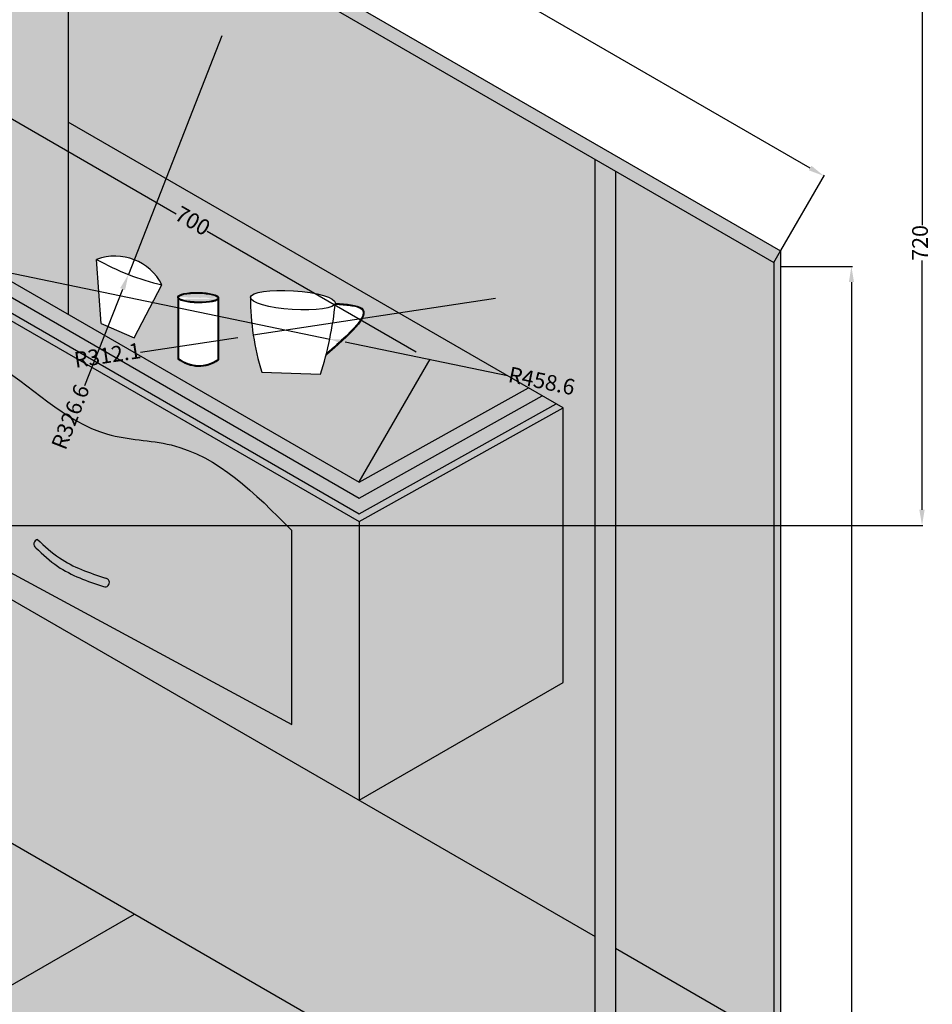
# Model space of a CAD drawing. Units: millimetres. Extents: x 78378 to 86415, y 148682 to 152721.
# Tile 15 of 18: x 80806 to 81968, y 150495 to 151749. Entities that reach past the tile are written whole.
import ezdxf

# ---------------------------------------------------------------- set-up
doc = ezdxf.new("R2010")
doc.units = ezdxf.units.MM
for name, color, linetype, lineweight in [('A-ANNO-DIMS', 2, 'Continuous', 18), ('A-FURN', 4, 'Continuous', 25), ('A-FURN-PATT', 32, 'Continuous', 13)]:
    doc.layers.add(name, color=color, linetype=linetype, lineweight=lineweight)
doc.styles.get("Standard").update_dxf_attribs({"font": 'arial.ttf'})
doc.dimstyles.new('ISO-25', dxfattribs={"dimtxt": 20, "dimasz": 20, "dimexe": 1.25, "dimexo": 0.625, "dimtad": 0, "dimdec": 1, "dimtxsty": 'Standard', "dimcen": 2.5, "dimadec": 0, "dimazin": 0, "dimtfac": 1, "dimtdec": 1, "dimtmove": 0, "dimatfit": 3, "dimfxl": 1, "dimarcsym": 0})

# ---------------------------------------------------------------- blocks, each defined once
blk = doc.blocks.new('*D1')
at = {"layer": 'A-ANNO-DIMS', "color": 0, "lineweight": -2, "transparency": 16777216}
for p, q in [((81775.8, 151435), (81866.6, 151435)), ((81865.3, 151415), (81865.3, 150363.7)), ((81865.3, 149279), (81865.3, 150302.4)), ((81775.8, 149259), (81866.6, 149259))]:
    blk.add_line(p, q, dxfattribs=at)
at = {"layer": 'A-ANNO-DIMS', "color": 0, "transparency": 16777216}
for points in [[(81862, 151415), (81868.6, 151415), (81865.3, 151435)], [(81862, 149279), (81868.6, 149279), (81865.3, 149259)]]:
    blk.add_solid(points, dxfattribs=at)
at = {"layer": 'Defpoints', "color": 0, "transparency": 16777216}
for p in [(81775.2, 151435), (81775.2, 149259), (81865.3, 149259)]:
    blk.add_point(p, dxfattribs=at)
at = {"layer": 'A-ANNO-DIMS', "color": 0, "transparency": 16777216, "insert": (81865.3, 150333), "char_height": 20, "attachment_point": 5, "rotation": 90}
blk.add_mtext('2176', dxfattribs=at)
blk = doc.blocks.new('*D3')
at = {"layer": 'A-ANNO-DIMS', "color": 0, "lineweight": -2, "transparency": 16777216}
for p, q in [((80389.8, 152255.5), (80445.2, 152351.4)), ((80461.9, 152340.3), (81144.7, 151946.1)), ((81812.9, 151560.3), (81195.8, 151916.6)), ((81775.5, 151455.5), (81830.8, 151551.4))]:
    blk.add_line(p, q, dxfattribs=at)
at = {"layer": 'A-ANNO-DIMS', "color": 0, "transparency": 16777216}
for points in [[(80463.5, 152343.2), (80460.2, 152337.4), (80444.5, 152350.3)], [(81814.5, 151563.2), (81811.2, 151557.4), (81830.2, 151550.3)]]:
    blk.add_solid(points, dxfattribs=at)
at = {"layer": 'Defpoints', "color": 0, "transparency": 16777216}
for p in [(80389.5, 152255), (81830.2, 151550.3), (81775.2, 151455)]:
    blk.add_point(p, dxfattribs=at)
at = {"layer": 'A-ANNO-DIMS', "color": 0, "transparency": 16777216, "insert": (81170.2, 151931.4), "char_height": 20, "attachment_point": 5, "rotation": 330}
blk.add_mtext('1600', dxfattribs=at)
blk = doc.blocks.new('*D30')
at = {"layer": 'A-ANNO-DIMS', "color": 0, "lineweight": -2, "transparency": 16777216}
for p, q in [((80615.3, 151825), (81956.4, 151825)), ((81955.2, 151805), (81955.2, 151487.6)), ((81955.2, 151125), (81955.2, 151442.4)), ((80615.3, 151105), (81956.4, 151105))]:
    blk.add_line(p, q, dxfattribs=at)
at = {"layer": 'A-ANNO-DIMS', "color": 0, "transparency": 16777216}
for points in [[(81951.8, 151805), (81958.5, 151805), (81955.2, 151825)], [(81951.8, 151125), (81958.5, 151125), (81955.2, 151105)]]:
    blk.add_solid(points, dxfattribs=at)
at = {"layer": 'Defpoints', "color": 0, "transparency": 16777216}
for p in [(80614.7, 151825), (81955.2, 151825), (80614.7, 151105)]:
    blk.add_point(p, dxfattribs=at)
at = {"layer": 'A-ANNO-DIMS', "color": 0, "transparency": 16777216, "insert": (81955.2, 151465), "char_height": 20, "attachment_point": 5, "rotation": 90}
blk.add_mtext('720', dxfattribs=at)
blk = doc.blocks.new('*D31')
at = {"layer": 'A-ANNO-DIMS', "color": 0, "lineweight": -2, "transparency": 16777216}
for p, q in [((80632.3, 151510.5), (80722.6, 151667)), ((80739.3, 151655.9), (81005.5, 151502.2)), ((81310.9, 151325.9), (81044.7, 151479.6)), ((81238.5, 151160.5), (81328.8, 151317))]:
    blk.add_line(p, q, dxfattribs=at)
at = {"layer": 'A-ANNO-DIMS', "color": 0, "transparency": 16777216}
for points in [[(80741, 151658.8), (80737.7, 151653), (80722, 151665.9)], [(81312.6, 151328.8), (81309.2, 151323), (81328.2, 151315.9)]]:
    blk.add_solid(points, dxfattribs=at)
at = {"layer": 'Defpoints', "color": 0, "transparency": 16777216}
for p in [(80632, 151510), (81328.2, 151315.9), (81238.2, 151160)]:
    blk.add_point(p, dxfattribs=at)
at = {"layer": 'A-ANNO-DIMS', "color": 0, "transparency": 16777216, "insert": (81025.1, 151490.9), "char_height": 20, "attachment_point": 5, "rotation": 330}
blk.add_mtext('700', dxfattribs=at)
blk = doc.blocks.new('*D69')
at = {"layer": 'A-ANNO-DIMS', "color": 0, "lineweight": -2, "transparency": 16777216}
for p, q in [((80751.9, 151435.6), (81200.9, 151342.5)), ((81427.3, 151295.6), (81220.5, 151338.5))]:
    blk.add_line(p, q, dxfattribs=at)
at = {"layer": 'A-ANNO-DIMS', "color": 0, "transparency": 16777216}
blk.add_solid([(81221.2, 151341.8), (81219.8, 151335.2), (81200.9, 151342.5)], dxfattribs=at)
at = {"layer": 'Defpoints', "color": 0, "transparency": 16777216}
for p in [(80751.9, 151435.6), (81200.9, 151342.5)]:
    blk.add_point(p, dxfattribs=at)
at = {"layer": 'A-ANNO-DIMS', "color": 0, "transparency": 16777216, "insert": (81470.4, 151286.7), "char_height": 20, "attachment_point": 5, "rotation": 348.2906}
blk.add_mtext('R458.6', dxfattribs=at)
blk = doc.blocks.new('*D70')
at = {"layer": 'A-ANNO-DIMS', "color": 0, "lineweight": -2, "transparency": 16777216}
for p, q in [((81063.6, 151728.9), (80944.5, 151424.8)), ((80889.1, 151283.3), (80937.2, 151406.2))]:
    blk.add_line(p, q, dxfattribs=at)
at = {"layer": 'A-ANNO-DIMS', "color": 0, "transparency": 16777216}
blk.add_solid([(80934.1, 151407.4), (80940.3, 151405), (80944.5, 151424.8)], dxfattribs=at)
at = {"layer": 'Defpoints', "color": 0, "transparency": 16777216}
for p in [(81063.6, 151728.9), (80944.5, 151424.8)]:
    blk.add_point(p, dxfattribs=at)
at = {"layer": 'A-ANNO-DIMS', "color": 0, "transparency": 16777216, "insert": (80873, 151242.4), "char_height": 20, "attachment_point": 5, "rotation": 68.6084}
blk.add_mtext('R326.6', dxfattribs=at)
blk = doc.blocks.new('*D71')
at = {"layer": 'A-ANNO-DIMS', "color": 0, "lineweight": -2, "transparency": 16777216}
for p, q in [((81412.1, 151394), (81103.5, 151347.4)), ((80959.9, 151325.7), (81083.7, 151344.4))]:
    blk.add_line(p, q, dxfattribs=at)
at = {"layer": 'A-ANNO-DIMS', "color": 0, "transparency": 16777216}
blk.add_solid([(81083.2, 151347.7), (81084.2, 151341.1), (81103.5, 151347.4)], dxfattribs=at)
at = {"layer": 'Defpoints', "color": 0, "transparency": 16777216}
for p in [(81412.1, 151394), (81103.5, 151347.4)]:
    blk.add_point(p, dxfattribs=at)
at = {"layer": 'A-ANNO-DIMS', "color": 0, "transparency": 16777216, "insert": (80918.3, 151319.4), "char_height": 20, "attachment_point": 5, "rotation": 8.593}
blk.add_mtext('R312.1', dxfattribs=at)

msp = doc.modelspace()

# ---------------------------------------------------------------- hatches: boundary and pattern name
at = {"layer": 'A-FURN-PATT'}
h = msp.add_hatch(color=256, dxfattribs=at)
h.dxf.hatch_style = 1
h.paths.add_polyline_path([(78839.3276, 151040.0076), (78579.52, 151190.0076), (78579.52, 150470.0076), (78839.3276, 150320.0076)])
h.paths.add_polyline_path([(79073.1545, 150899.6469, 0.277779695), (79002.2645, 150996.3205, 0.791083931), (78917.9567, 150978.8719, 0.180448316), (78856.6481, 150853.0138), (78856.6481, 150350.6973), (79073.1545, 150484.318)])
h.paths.add_polyline_path([(79073.1545, 151175.0076), (78856.6481, 151050.0076), (78856.6481, 150853.0138, -0.180448316), (78917.9567, 150978.8719, -0.791083931), (79002.2645, 150996.3205, -0.277779695), (79073.1545, 150899.6469)])
h.paths.add_polyline_path([(79341.6224, 151350.0076), (79099.1352, 151490.0076), (78596.8405, 151200.0076), (78839.3276, 151060.0076)])
h.paths.add_polyline_path([(79904.5389, 151675.0076), (79662.0518, 151815.0076), (79099.1352, 151490.0076), (79341.6224, 151350.0076)])
h.paths.add_polyline_path([(80389.5131, 151955.0076), (80389.5131, 152235.0076), (79662.0518, 151815.0076), (79904.5389, 151675.0076)])
h.paths.add_polyline_path([(80389.5131, 151955.0076), (80164.3465, 151825.0076), (80164.3465, 151105.0076), (80614.6797, 151105.0076), (80614.6797, 151825.0076)])
edge = h.paths.add_edge_path(flags=16)
edge.add_spline(control_points=[(80216.308, 151728.251), (80227.1854, 151732.981), (80256.3301, 151745.6544), (80298.41, 151761.9595), (80340.2597, 151805.855), (80391.0771, 151782.0404), (80454.0396, 151805.7581), (80496.5007, 151742.4095), (80543.8218, 151733.4043), (80562.7182, 151729.8083)], knot_values=[0, 0, 0, 0, 35.543746761, 95.235753469, 136.367675126, 200.932981967, 236.726410811, 322.889934976, 380.170273667, 380.170273667, 380.170273667, 380.170273667], degree=3, periodic=0)
edge.add_line((80562.7182, 151729.8083), (80562.7182, 151165.0076))
edge.add_line((80562.7182, 151165.0076), (80216.308, 151165.0076))
edge.add_line((80216.308, 151165.0076), (80216.308, 151728.251))
h.paths.add_polyline_path([(80632.0002, 152095.0076), (80389.5131, 152235.0076), (80389.5131, 151955.0076), (80614.6797, 151825.0076), (80632.0002, 151815.0076)])
h.paths.add_polyline_path([(80867.7794, 151958.8805), (80632.0002, 152095.0076), (80632.0002, 151815.0076), (80632.0002, 151510.0076), (80867.7794, 151373.8805)])
h.paths.add_polyline_path([(80147.026, 151495.8203, 0.18918979), (80063.5671, 151597.7244, 0.788261355), (79979.2691, 151580.5832, 0.160726132), (79904.5389, 151413.5769), (79904.5389, 150955.0076), (80147.026, 151095.0076)])
h.paths.add_polyline_path([(80147.026, 151815.0076), (79904.5389, 151675.0076), (79904.5389, 151413.5769, -0.160726132), (79979.2691, 151580.5832, -0.788261355), (80063.5671, 151597.7244, -0.18918979), (80147.026, 151495.8203)])
h.paths.add_polyline_path([(79887.2184, 151645.0076), (79640.4011, 151502.5076), (79640.4011, 151262.3325, -0.160726132), (79715.1313, 151429.3387, -0.788261355), (79799.4294, 151446.48, -0.21290578), (79887.2184, 151328.7247)])
h.paths.add_polyline_path([(79799.4294, 151446.48, 0.788261355), (79715.1313, 151429.3387, 0.160726132), (79640.4011, 151262.3325), (79640.4011, 150822.5076), (79887.2184, 150965.0076), (79887.2184, 151328.7247, 0.21290578)])
h.paths.add_polyline_path([(79605.7601, 151482.5076), (79358.9429, 151340.0076), (79358.9429, 151100.0701, -0.160726132), (79433.6731, 151267.0764, -0.788261355), (79517.9711, 151284.2176, -0.21290578), (79605.7601, 151166.4623)])
h.paths.add_polyline_path([(79605.7601, 151166.4623, 0.21290578), (79517.9711, 151284.2176, 0.788261355), (79433.6731, 151267.0764, 0.160726132), (79358.9429, 151100.0701), (79358.9429, 150742.9831), (79419.0877, 150694.7323), (79605.7601, 150802.5076)])
edge = h.paths.add_edge_path(flags=0)
edge.add_spline(control_points=[(81152.4356, 151098.7676), (81105.7208, 151145.9466), (81038.6136, 151213.7208), (80882.3866, 151214.1938), (80797.4434, 151311.2997), (80711.8686, 151340.3754), (80681.7691, 151350.6023)], knot_values=[0, 0, 0, 0, 188.233441, 270.4032752, 445.451792012, 540.428588287, 540.428588287, 540.428588287, 540.428588287], degree=3, periodic=0)
edge.add_line((80683.4538, 151350.0269), (80683.4538, 151104.8792))
edge.add_line((80683.4538, 151104.8792), (81152.4356, 150851.399))
edge.add_line((81152.4356, 150851.399), (81152.4356, 151098.7676))
edge = h.paths.add_edge_path(flags=0)
edge.add_spline(control_points=[(80912.9018, 151027.1103), (80892.3742, 151034.1027), (80860.1663, 151045.0739), (80835.5097, 151068.1214), (80826.5679, 151076.4797)], knot_values=[0, 0, 0, 0, 63.98405104, 100.391424282, 100.391424282, 100.391424282, 100.391424282], degree=3, periodic=0)
edge.add_arc((80830.0414, 151081.2992), 5.9407, 100.9277276, 234.2187381, ccw=False)
edge.add_spline(control_points=[(80828.9152, 151087.1322), (80837.857, 151078.7739), (80862.5136, 151055.7263), (80894.7215, 151044.7552), (80915.2491, 151037.7628)], knot_values=[0, 0, 0, 0, 36.407373242, 100.391424282, 100.391424282, 100.391424282, 100.391424282], degree=3, periodic=0)
edge.add_arc((80914.7882, 151032.2795), 5.5026, -107.9540399, 85.195579, ccw=False)
h.paths.add_polyline_path([(81238.218, 151110.0076), (80632.0002, 151460.0076), (80632.0002, 151105.0076), (81238.218, 150755.0076)])
edge = h.paths.add_edge_path(flags=16)
edge.add_line((81152.4356, 150851.399), (80683.4538, 151104.8792))
edge.add_line((80683.4538, 151104.8792), (80683.4538, 151350.0279))
edge.add_spline(control_points=[(80681.7691, 151350.6023), (80711.8686, 151340.3754), (80797.4434, 151311.2997), (80882.3866, 151214.1938), (81038.6136, 151213.7208), (81105.7208, 151145.9466), (81152.4356, 151098.7676)], knot_values=[0, 0, 0, 0, 94.976796275, 270.025313088, 352.195147288, 540.428588287, 540.428588287, 540.428588287, 540.428588287], degree=3, periodic=0)
edge.add_line((81152.4356, 151098.7676), (81152.4356, 150851.399))
edge = h.paths.add_edge_path(flags=0)
edge.add_spline(control_points=[(80912.9018, 151027.1103), (80892.3742, 151034.1027), (80860.1663, 151045.0739), (80835.5097, 151068.1214), (80826.5679, 151076.4797)], knot_values=[0, 0, 0, 0, 63.98405104, 100.391424282, 100.391424282, 100.391424282, 100.391424282], degree=3, periodic=0)
edge.add_arc((80830.0414, 151081.2992), 5.9407, 100.9277276, 234.2187381, ccw=False)
edge.add_spline(control_points=[(80828.9152, 151087.1322), (80837.857, 151078.7739), (80862.5136, 151055.7263), (80894.7215, 151044.7552), (80915.2491, 151037.7628)], knot_values=[0, 0, 0, 0, 36.407373242, 100.391424282, 100.391424282, 100.391424282, 100.391424282], degree=3, periodic=0)
edge.add_arc((80914.7882, 151032.2795), 5.5026, -107.7417882, 85.195579, ccw=False)
h.paths.add_polyline_path([(81498.0256, 151255.0076), (81238.218, 151110.0076), (81238.218, 150755.0076), (81498.0256, 150905.0076)])
edge = h.paths.add_edge_path(flags=16)
edge.add_spline(control_points=[(81152.4356, 151098.7676), (81105.7208, 151145.9466), (81038.6136, 151213.7208), (80882.3866, 151214.1938), (80797.4434, 151311.2997), (80711.8686, 151340.3754), (80681.7691, 151350.6023)], knot_values=[0, 0, 0, 0, 188.233441, 270.4032752, 445.451792012, 540.428588287, 540.428588287, 540.428588287, 540.428588287], degree=3, periodic=0)
edge.add_line((80683.4538, 151350.0279), (80683.4538, 151104.8792))
edge.add_line((80683.4538, 151104.8792), (81152.4356, 150851.399))
edge.add_line((81152.4356, 150851.399), (81152.4356, 151098.7676))
h.paths.add_polyline_path([(81453.9904, 151280.4314), (80867.7794, 151618.8805), (80867.7794, 151373.8805), (81238.218, 151160.0076)])
edge = h.paths.add_edge_path(flags=16)
edge.add_line((81189.2304, 151297.6373), (81114.4166, 151300.2154))
edge.add_arc((81412.0967, 151394.0167), 312.1092, 179.7569303, 197.4900342, ccw=False)
edge.add_ellipse((81154.0183, 151392.0436), major_axis=(-54.0264, 3.6301), ratio=0.221796934, start_angle=0, end_angle=0.3517985, ccw=False)
edge.add_ellipse((81154.0183, 151392.0436), major_axis=(-54.0264, 3.6301), ratio=0.221796934, start_angle=180, end_angle=360, ccw=False)
edge.add_spline(control_points=[(81196.1844, 151321.9476), (81224.9802, 151347.1455), (81266.8846, 151383.8144), (81222.0354, 151387.0304), (81208.0056, 151388.0364)], knot_values=[0, 0, 0, 0, 75.091751734, 109.275804387, 109.275804387, 109.275804387, 109.275804387], degree=3, periodic=0)
edge.add_arc((80751.9112, 151435.6145), 458.5693, 342.4891602, 345.646172, ccw=False)
edge = h.paths.add_edge_path(flags=0)
edge.add_spline(control_points=[(81196.6193, 151323.657), (81197.893, 151324.7717), (81199.1654, 151325.8858), (81209.0233, 151334.5343), (81217.3959, 151341.9835), (81228.0928, 151352.5012), (81231.3883, 151355.9524), (81236.9493, 151362.4395), (81239.214, 151365.4773), (81241.4987, 151369.416), (81242.064, 151370.5542), (81242.9187, 151372.6971), (81243.2076, 151373.7015), (81243.5012, 151375.5539), (81243.5065, 151376.4), (81243.2432, 151377.9407), (81242.9775, 151378.6373), (81242.1402, 151379.937), (81241.5659, 151380.5416), (81240.2039, 151381.533), (81239.4963, 151381.9384), (81237.0619, 151383.0663), (81235.0242, 151383.6999), (81230.352, 151384.7569), (81227.7173, 151385.1826), (81221.9118, 151385.9145), (81218.7193, 151386.2133), (81213.7912, 151386.6115), (81212.1252, 151386.7359), (81209.6196, 151386.9181), (81208.7865, 151386.9779), (81207.9009, 151387.0432)], knot_values=[0.015487437, 0.015487437, 0.015487437, 0.015487437, 3.337879569, 3.337879569, 25.851306242, 25.851306242, 37.52811308, 37.52811308, 49.204919918, 49.204919918, 54.285093801, 54.285093801, 59.365267683, 59.365267683, 64.445441566, 64.445441566, 69.525615449, 69.525615449, 74.605789331, 74.605789331, 78.493667847, 78.493667847, 86.255670953, 86.255670953, 94.017674059, 94.017674059, 102.202265559, 102.202265559, 106.294561309, 106.294561309, 108.325221747, 108.325221747, 108.325221747, 108.325221747], degree=3, periodic=0)
edge = h.paths.add_edge_path(flags=16)
edge.add_arc((81034.1732, 151350.4693), 42.5822, 231.2679035, 306.151846, ccw=False)
edge.add_line((81007.5303, 151317.2517), (81007.5303, 151395.181))
edge.add_ellipse((81033.412, 151394.7791), major_axis=(-25.8816, 0.4538), ratio=0.23894509, start_angle=0, end_angle=0.1147075, ccw=False)
edge.add_ellipse((81033.412, 151394.7791), major_axis=(-25.8816, 0.4538), ratio=0.23894509, start_angle=181.1677709, end_angle=358.9476457, ccw=False)
edge.add_ellipse((81033.412, 151395.7791), major_axis=(-25.8816, 0.4538), ratio=0.23894509, start_angle=180, end_angle=360.1147075, ccw=False)
edge.add_ellipse((81033.412, 151395.7791), major_axis=(-25.8816, 0.4538), ratio=0.23894509, start_angle=178.9476457, end_angle=180, ccw=False)
edge.add_line((81059.2936, 151395.1778), (81059.2936, 151394.3772))
edge.add_ellipse((81033.412, 151394.7791), major_axis=(-25.8816, 0.4538), ratio=0.23894509, start_angle=180, end_angle=180.1147075, ccw=False)
edge.add_ellipse((81033.412, 151394.7791), major_axis=(-25.8816, 0.4538), ratio=0.23894509, start_angle=3.6903098, end_angle=176.4406503, ccw=False)
edge.add_line((81059.2936, 151393.3388), (81059.2936, 151316.086))
h.paths.add_polyline_path([(80951.9355, 151343.9568), (80909.6838, 151362.4635), (80904.0219, 151443.9615, -0.381333076), (80987.2169, 151411.3717)], flags=16)
h = msp.add_hatch(color=256, dxfattribs=at)
h.dxf.hatch_style = 1
h.paths.add_polyline_path([(80867.7794, 151978.8805), (80867.7794, 151958.8805), (81766.4935, 151440.0076), (81766.4935, 150140.0076), (81775.1537, 150135.0076), (81775.1537, 151455.0076)])
h = msp.add_hatch(color=256, dxfattribs=at)
h.dxf.hatch_style = 1
h.paths.add_polyline_path([(80389.8136, 150935.1811), (80389.5131, 151105.0076), (80164.3465, 151105.0076), (79904.5389, 150955.0076), (79433.5848, 150683.1022), (79459.4128, 150662.3818), (79243.9048, 150537.9582), (79160.4069, 150518.1674), (78839.3276, 150320.0076), (78579.52, 150470.0076), (78570.8597, 150475.0076), (78570.8597, 150465.0076), (78570.8597, 149885.0076)])
h.paths.add_polyline_path([(80086.4042, 150460.0076), (79826.5966, 150610.0076), (78570.8597, 149885.0076), (78830.6674, 149735.0076)])
h.paths.add_polyline_path([(79540.8001, 150161.0557), (79217.3967, 149974.3386), (78980.9166, 150110.8705), (79304.32, 150297.5875)], flags=16)
h.paths.add_polyline_path([(79506.159, 150161.0557), (79217.3967, 149994.3386), (79015.5576, 150110.8705), (79304.32, 150277.5875)], flags=0)
edge = h.paths.add_edge_path(flags=0)
edge.add_arc((79247.8636, 150177.1541), 137.9799, 256.0025928, 293.5594109)
edge.add_arc((79240.7671, 150078.2605), 68.0855, 336.099104, 387.3696877)
edge.add_ellipse((79258.3074, 150109.4852), major_axis=(-42.6234, -1.6591), ratio=0.160428429, start_angle=0, end_angle=179.0977279, ccw=False)
edge.add_arc((79285.2112, 150074.2509), 77.2096, 155.1233104, 203.6557939)
edge = h.paths.add_edge_path(flags=0)
edge.add_ellipse((79258.6958, 150110.8297), major_axis=(-42.6234, -1.6591), ratio=0.160428429, start_angle=350.6039412, end_angle=356.2289762)
edge.add_line((79219.169, 150111.8937), (79218.3268, 150109.4141))
edge.add_arc((79262.4675, 150032.9602), 88.2813, 112.3931229, 120, ccw=False)
h.paths.add_polyline_path([(79287.0625, 150086.9703, -0.247702064), (79288.1967, 150077.2955, -0.390476513), (79265.4731, 150072.5438, -0.487261526), (79264.079, 150082.3769, 0.395604326)], flags=0)
h.paths.add_polyline_path([(80389.5131, 150935.0076), (79826.5966, 150610.0076), (80086.4042, 150460.0076), (80692.622, 150460.0076), (80952.4296, 150610.0076)])
edge = h.paths.add_edge_path(flags=16)
edge.add_ellipse((80392.4466, 150825.601), major_axis=(-133.0757, 7.722), ratio=0.42449957, start_angle=0, end_angle=360)
edge = h.paths.add_edge_path(flags=0)
edge.add_spline(control_points=[(80269.3541, 150832.7436), (80269.2919, 150831.672), (80269.3503, 150830.5922), (80269.7341, 150828.3361), (80270.0612, 150827.1587), (80271.0461, 150824.6748), (80271.7052, 150823.3692), (80273.4061, 150820.6503), (80274.4481, 150819.2381), (80276.9366, 150816.3509), (80278.3828, 150814.8762), (80282.5858, 150811.0913), (80285.6261, 150808.7701), (80292.6031, 150804.2267), (80296.5388, 150802.0041), (80305.195, 150797.7581), (80309.9151, 150795.7344), (80320.0112, 150791.96), (80325.387, 150790.2092), (80339.2162, 150786.315), (80347.9578, 150784.3563), (80366.0679, 150781.2568), (80375.4359, 150780.1158), (80394.3093, 150778.7158), (80403.8142, 150778.4568), (80422.4656, 150778.8319), (80431.6115, 150779.4662), (80449.0608, 150781.5838), (80457.3636, 150783.0675), (80472.6699, 150786.7766), (80479.6726, 150789.0033), (80490.1894, 150793.2813), (80494.1268, 150795.1967), (80501.0146, 150799.1885), (80503.9632, 150801.2651), (80508.2066, 150804.9015), (80509.73, 150806.4609), (80512.1996, 150809.4942), (80513.1456, 150810.9657), (80514.4291, 150813.5431), (80514.8436, 150814.6688), (80515.3984, 150816.8625), (80515.5405, 150817.9315), (80515.5801, 150820.098), (80515.4773, 150821.1978), (80514.9905, 150823.5062), (80514.6047, 150824.7154), (80513.4854, 150827.2641), (80512.7511, 150828.6027), (80510.8872, 150831.3809), (80509.7578, 150832.8196), (80507.0873, 150835.7513), (80505.5466, 150837.2439), (80501.0624, 150841.0944), (80497.8199, 150843.4576), (80490.4174, 150848.062), (80486.2582, 150850.3037), (80477.1448, 150854.5643), (80472.1909, 150856.5835), (80461.6275, 150860.3245), (80456.0182, 150862.0465), (80441.7332, 150865.8127), (80432.7885, 150867.6675), (80414.3391, 150870.5317), (80404.8349, 150871.5411), (80385.7707, 150872.6572), (80376.2113, 150872.764), (80357.5444, 150872.0728), (80348.4375, 150871.2748), (80331.1682, 150868.83), (80323.0064, 150867.1827), (80309.472, 150863.5363), (80303.8628, 150861.6593), (80293.8018, 150857.5401), (80289.3512, 150855.2969), (80282.7757, 150851.2345), (80280.3473, 150849.4579), (80276.2606, 150845.9127), (80274.604, 150844.1458), (80272.3157, 150841.1243), (80271.5358, 150839.8454), (80270.3496, 150837.3879), (80269.9417, 150836.2101), (80269.5065, 150834.2815), (80269.3988, 150833.5143), (80269.3541, 150832.7436)], knot_values=[0, 0, 0, 0, 0.09750046, 0.09750046, 0.19500092, 0.19500092, 0.292501379, 0.292501379, 0.390001839, 0.390001839, 0.487502299, 0.487502299, 0.638803224, 0.638803224, 0.790104149, 0.790104149, 0.941405074, 0.941405074, 1.092705999, 1.092705999, 1.312817101, 1.312817101, 1.532928203, 1.532928203, 1.753039304, 1.753039304, 1.973150406, 1.973150406, 2.193261508, 2.193261508, 2.413372609, 2.413372609, 2.569860633, 2.569860633, 2.726348657, 2.726348657, 2.844186582, 2.844186582, 2.962024507, 2.962024507, 3.060233876, 3.060233876, 3.158443245, 3.158443245, 3.256652615, 3.256652615, 3.354861984, 3.354861984, 3.453071354, 3.453071354, 3.551280723, 3.551280723, 3.649490093, 3.649490093, 3.80392773, 3.80392773, 3.958365368, 3.958365368, 4.112803006, 4.112803006, 4.267240644, 4.267240644, 4.489203495, 4.489203495, 4.711166346, 4.711166346, 4.933129197, 4.933129197, 5.155092048, 5.155092048, 5.3770549, 5.3770549, 5.557853609, 5.557853609, 5.738652318, 5.738652318, 5.872395556, 5.872395556, 6.006138794, 6.006138794, 6.109604996, 6.109604996, 6.213071198, 6.213071198, 6.283185307, 6.283185307, 6.283185307, 6.283185307], degree=3, periodic=0)
edge = h.paths.add_edge_path(flags=0)
edge.add_ellipse((80392.4466, 150825.601), major_axis=(-101.8398, 3.3923), ratio=0.403492477, start_angle=0, end_angle=360)
edge = h.paths.add_edge_path(flags=0)
edge.add_ellipse((80391.1657, 150858.3746), major_axis=(9.0882, -0.6733), ratio=0.351354129, start_angle=0, end_angle=360)
h.paths.add_polyline_path([(80952.4296, 150610.0076), (80692.622, 150460.0076), (81361.2342, 150073.9842), (81649.9628, 150052.7286), (81766.4935, 150120.0076), (81766.4935, 150140.0076), (81564.9025, 150256.3963), (81564.8884, 150096.1963), (81538.9076, 150111.1963), (81538.9217, 150271.3963)])
h.paths.add_polyline_path([(81539.0357, 151571.3305), (80867.7794, 151958.8805), (80867.7794, 151618.8805), (81498.0256, 151255.0076), (81498.0256, 150905.0076), (81238.218, 150755.0076), (81538.9488, 150581.3806)])
h.paths.add_polyline_path([(81766.4935, 151440.0076), (81565.0164, 151556.3305), (81564.9296, 150566.3806), (81766.4935, 150450.0076)])
edge = h.paths.add_edge_path()
edge.add_line((81564.9296, 150566.3806), (81564.9137, 150384.6289))
edge.add_ellipse((81552.1304, 150358.5718), major_axis=(52.6272, 3.506), ratio=0.495899055, start_angle=367.5169757, end_angle=420.0564686, ccw=False)
edge.add_ellipse((81552.1304, 150358.5718), major_axis=(52.6272, 3.506), ratio=0.495899055, start_angle=351.729742, end_angle=367.5169757, ccw=False)
edge.add_ellipse((81552.1304, 150345.5016), major_axis=(52.6272, 3.506), ratio=0.495899055, start_angle=352.5116949, end_angle=366.3006092, ccw=False)
edge.add_line((81603.4463, 150342.2039), (81603.5064, 150340.4475))
edge.add_ellipse((81552.1304, 150332.128), major_axis=(52.6272, 3.506), ratio=0.495899055, start_angle=353.6729654, end_angle=365.3867997, ccw=False)
edge.add_ellipse((81552.1304, 150332.128), major_axis=(52.6272, 3.506), ratio=0.495899055, start_angle=350.9388331, end_angle=353.6729654)
edge.add_line((81603.8688, 150329.855), (81604.0442, 150324.7302))
edge.add_ellipse((81552.1304, 150317.7418), major_axis=(52.6272, 3.506), ratio=0.495899055, start_angle=355.2176746, end_angle=363.8553364, ccw=False)
edge.add_ellipse((81552.1304, 150317.7418), major_axis=(52.6272, 3.506), ratio=0.495899055, start_angle=341.3250873, end_angle=355.2176746, ccw=False)
edge.add_ellipse((81552.1304, 150317.7418), major_axis=(52.6272, 3.506), ratio=0.495899055, start_angle=293.4661701, end_angle=341.3250873, ccw=False)
edge.add_line((81564.9057, 150292.9664), (81564.9025, 150256.3963))
edge.add_line((81564.9025, 150256.3963), (81766.4935, 150140.0076))
edge.add_line((81766.4935, 150140.0076), (81766.4935, 150450.0076))
edge.add_line((81766.4935, 150450.0076), (81564.9296, 150566.3806))
h.paths.add_polyline_path([(81525.5713, 150321.598), (81526.5985, 150321.3069), (81528.6771, 150320.947)])
h.paths.add_polyline_path([(81512.7903, 150326.1129), (81514.5058, 150325.3887), (81512.538, 150326.2678)])
h.paths.add_polyline_path([(81533.2148, 150320.1615), (81534.6952, 150319.9052), (81536.5995, 150319.7557)])
h.paths.add_polyline_path([(81518.622, 150323.6513), (81519.227, 150323.3959), (81521.289, 150322.8116)])
h.paths.add_polyline_path([(81501.2183, 150336.2599), (81500.3543, 150338.1339), (81499.7815, 150340.0494), (81499.5032, 150341.9955), (81499.5032, 150343.7257), (81499.7584, 150345.5905), (81500.2766, 150347.4549), (81501.0551, 150349.3095), (81501.0967, 150349.3937), (81501.1389, 150349.4778), (81500.9978, 150349.7496), (81500.8628, 150350.0225), (81499.5032, 150355.0658), (81499.9591, 150359.5002), (81501.8982, 150363.9083), (81505.2653, 150368.1646), (81509.9647, 150372.1482), (81515.8627, 150375.7459), (81522.7918, 150378.8553), (81530.555, 150381.3882), (81538.9315, 150383.2724), (81538.9488, 150581.3806), (80632.0002, 151105.0076), (80389.5131, 151105.0076), (80389.8142, 150934.8338), (80952.4296, 150610.0076), (81538.9217, 150271.3963), (81538.9234, 150291.7194), (81538.8752, 150291.721), (81530.1915, 150292.8239), (81522.1802, 150294.6904), (81515.0866, 150297.2633), (81509.8635, 150299.9959), (81505.6084, 150303.1351), (81502.419, 150306.6088), (81500.3683, 150310.3375), (81499.5032, 150314.2358), (81499.5032, 150315.9659), (81499.8206, 150318.1159), (81500.487, 150320.2634), (81501.4979, 150322.3941), (81500.487, 150324.4233), (81499.8206, 150326.5039), (81499.5032, 150328.622), (81499.5032, 150330.3521), (81499.7815, 150332.3262), (81500.3543, 150334.2992)])
h = msp.add_hatch(color=256, dxfattribs=at)
h.dxf.hatch_style = 1
h.paths.add_polyline_path([(79090.475, 151205.0076), (78839.3276, 151060.0076), (78839.3276, 150320.0076), (79090.475, 150475.0076)])
h.paths.add_polyline_path([(79073.1545, 151175.0076), (79073.1545, 150899.6469, -0.04544363), (79073.1545, 150878.5653), (79073.1545, 150484.318), (78856.6481, 150350.6973), (78856.6481, 150814.5249, -0.048157161), (78856.6481, 150853.0138), (78856.6481, 151050.0076)], flags=16)
h.paths.add_polyline_path([(79358.9429, 151340.0076), (79605.7601, 151482.5076), (79605.7601, 150802.5076), (79419.0877, 150694.7323), (79433.5848, 150683.1022), (79623.0806, 150792.5076), (79623.0806, 151512.5076), (79341.6224, 151350.0076), (79341.6224, 150756.8784), (79358.9429, 150742.9831)])
h.paths.add_polyline_path([(79341.6224, 151350.0076), (79090.475, 151205.0076), (79090.475, 150475.0076), (79160.4069, 150518.1674), (79107.7955, 150505.6973), (79107.7955, 151195.0076), (79109.5275, 151196.0076), (79324.3018, 151320.0076), (79324.3018, 150770.7736), (79341.6224, 150756.8784)])
h.paths.add_polyline_path([(79887.2184, 151645.0076), (79887.2184, 151665.0076), (79623.0806, 151512.5076), (79623.0806, 150792.5076), (79887.2184, 150945.0076), (79887.2184, 150965.0076), (79640.4011, 150822.5076), (79640.4011, 151502.5076)])
h.paths.add_polyline_path([(79904.5389, 151655.0076), (79887.2184, 151645.0076), (79887.2184, 150965.0076), (79904.5389, 150975.0076)])
h.paths.add_polyline_path([(80164.3465, 151825.0076), (80147.026, 151815.0076), (80147.026, 151095.0076), (80164.3465, 151105.0076)])
h.paths.add_polyline_path([(80632.0002, 151510.0076), (80632.0002, 151490.0076), (81238.218, 151140.0076), (81471.6045, 151270.2619), (81453.9904, 151280.4314), (81238.218, 151160.0076)])
h.paths.add_polyline_path([(80632.0002, 151490.0076), (80632.0002, 151470.0076), (81238.218, 151120.0076), (81489.2186, 151260.0924), (81471.6045, 151270.2619), (81238.218, 151140.0076)])
h.paths.add_polyline_path([(80632.0002, 151460.0076), (80632.0002, 151105.0076), (81238.218, 150755.0076), (81238.218, 151110.0076)])
edge = h.paths.add_edge_path(flags=16)
edge.add_spline(control_points=[(80681.7691, 151350.6023), (80711.8686, 151340.3754), (80797.4434, 151311.2997), (80882.3866, 151214.1938), (81038.6136, 151213.7208), (81105.7208, 151145.9466), (81152.4356, 151098.7676)], knot_values=[0, 0, 0, 0, 94.976796275, 270.025313088, 352.195147288, 540.428588287, 540.428588287, 540.428588287, 540.428588287], degree=3, periodic=0)
edge.add_line((81152.4356, 151098.7676), (81152.4356, 150851.399))
edge.add_line((81152.4356, 150851.399), (80683.4538, 151104.8792))
edge.add_line((80683.4538, 151104.8792), (80683.4538, 151350.027))
edge = h.paths.add_edge_path(flags=0)
edge.add_spline(control_points=[(80828.9152, 151087.1322), (80837.857, 151078.7739), (80862.5136, 151055.7263), (80894.7215, 151044.7552), (80915.2491, 151037.7628)], knot_values=[0, 0, 0, 0, 36.407373242, 100.391424282, 100.391424282, 100.391424282, 100.391424282], degree=3, periodic=0)
edge.add_arc((80914.7882, 151032.2795), 5.5026, -107.9540399, 85.195579, ccw=False)
edge.add_spline(control_points=[(80912.9018, 151027.1103), (80892.3742, 151034.1027), (80860.1663, 151045.0739), (80835.5097, 151068.1214), (80826.5679, 151076.4797)], knot_values=[0, 0, 0, 0, 63.98405104, 100.391424282, 100.391424282, 100.391424282, 100.391424282], degree=3, periodic=0)
edge.add_arc((80830.0414, 151081.2992), 5.9407, 100.9277276, 234.2187381, ccw=False)
h.paths.add_polyline_path([(80632.0002, 151815.0076), (80614.6797, 151825.0076), (80614.6797, 151105.0076), (80632.0002, 151105.0076)])
h.paths.add_polyline_path([(81498.0256, 151255.0076), (81489.2186, 151260.0924), (81238.218, 151120.0076), (80632.0002, 151470.0076), (80632.0002, 151460.0076), (81238.218, 151110.0076)])
h.paths.add_polyline_path([(78596.8405, 151200.0076), (78579.52, 151190.0076), (78839.3276, 151040.0076), (78839.3276, 151060.0076)])
h.paths.add_polyline_path([(78596.8405, 151200.0076), (78579.52, 151210.0076), (78579.52, 151190.0076)])
h.paths.add_polyline_path([(78579.52, 151210.0076), (78570.8597, 151205.0076), (78570.8597, 150475.0076), (78579.52, 150470.0076)])
h = msp.add_hatch(color=256, dxfattribs=at)
h.dxf.hatch_style = 1
edge = h.paths.add_edge_path()
edge.add_line((81565.0164, 151556.3305), (81539.0357, 151571.3305))
edge.add_line((81539.0357, 151571.3305), (81538.927, 150332.5469))
edge.add_ellipse((81552.1304, 150358.5718), major_axis=(52.6272, 3.506), ratio=0.495899055, start_angle=239.2882719, end_angle=293.4732997)
edge.add_line((81564.9092, 150333.797), (81565.0164, 151556.3305))
edge = h.paths.add_edge_path()
edge.add_ellipse((81552.1304, 150317.7418), major_axis=(52.6272, 3.506), ratio=0.495899055, start_angle=239.2817509, end_angle=293.4661701, ccw=False)
edge.add_line((81538.9234, 150291.7172), (81538.9076, 150111.1963))
edge.add_line((81538.9076, 150111.1963), (81564.8884, 150096.1963))
edge.add_line((81564.8884, 150096.1963), (81564.9057, 150292.9664))

# ---------------------------------------------------------------- linework, layer by layer
at = {"layer": 'A-FURN'}
for p, q in [((80389.5131, 152255.0076), (81775.1537, 151455.0076)), ((80389.5131, 152235.0076), (81766.4935, 151440.0076)), ((80867.7794, 151958.8805), (80867.7794, 151373.8805)), ((81498.0256, 151255.0076), (80867.7794, 151618.8805)), ((81538.9076, 150111.7066), (81539.0357, 151571.3305)), ((81565.0164, 151556.3305), (81564.8884, 150096.1963)), ((80632.0002, 151510.0076), (81238.218, 151160.0076)), ((80632.0002, 151490.0076), (81238.218, 151140.0076)), ((80632.0002, 151470.0076), (81238.218, 151120.0076)), ((80632.0002, 151460.0076), (81238.218, 151110.0076)), ((81766.4935, 151440.0076), (81775.1537, 151455.0076)), ((81775.1537, 151455.0076), (81775.1537, 149259.0076)), ((80909.6838, 151362.4635), (80904.0219, 151443.9615)), ((81766.4935, 151440.0076), (81766.4935, 149264.0076)), ((80951.9355, 151343.9568), (80987.2169, 151411.3717)), ((81007.5303, 151396.181), (81007.5303, 151317.2517)), ((81008.3964, 151393.6056), (81008.3964, 151317.5753)), ((81058.4315, 151392.782), (81058.4315, 151316.4724)), ((81059.2936, 151395.3253), (81059.2936, 151316.086)), ((80909.6838, 151362.4635), (80951.9355, 151343.9568)), ((81114.4166, 151300.2154), (81189.2304, 151297.6373)), ((81238.218, 151160.0076), (81453.9904, 151280.4314)), ((81238.218, 151140.0076), (81471.6045, 151270.2619)), ((81238.218, 151120.0076), (81489.2186, 151260.0924)), ((81238.218, 151110.0076), (81498.0256, 151255.0076)), ((81498.0256, 150905.0076), (81498.0256, 151255.0076)), ((81539.0059, 151231.3477), (81539.0111, 151231.3446)), ((81238.218, 151110.0076), (81238.218, 150755.0076)), ((80632.0002, 151105.0076), (81538.9488, 150581.3806)), ((80683.4538, 151104.8792), (81152.4356, 150851.399)), ((81152.4356, 150851.399), (81152.4356, 151098.7676)), ((80389.5131, 150935.0076), (81538.9076, 150271.4044)), ((81238.218, 150755.0076), (81498.0256, 150905.0076)), ((80692.622, 150460.0076), (80952.4296, 150610.0076)), ((81564.9296, 150566.3806), (81766.4935, 150450.0076))]:
    msp.add_line(p, q, dxfattribs=at)
for centre, radius, start, end in [((80927.3606, 151381.0556), 67.0958, 26.8613413, 110.3553554), ((81063.6143, 151728.8832), 326.5733, 240.7456288, 256.4710679), ((81412.0967, 151394.0167), 312.1092, 179.6958002, 197.4900342), ((80751.9112, 151435.6145), 458.5693, 342.4891602, 354.0920293), ((81034.1732, 151350.4693), 42.5822, 231.2679035, 306.151846), ((81034.1732, 151351.4693), 42.5822, 232.7465418, 304.7280677), ((80830.0414, 151081.2992), 5.9407, 100.9277276, 234.2187381), ((80914.7882, 151032.2795), 5.5026, 249.9508867, 85.195579)]:
    msp.add_arc(centre, radius, start, end, dxfattribs=at)
for centre, major_axis, ratio in [((81033.412, 151395.7791), (-25.8816, 0.4538), 0.23894509), ((81033.412, 151394.7791), (-25.8816, 0.4538), 0.23894509), ((81154.0183, 151392.0436), (-54.0264, 3.6301), 0.221796934)]:
    msp.add_ellipse(centre, major_axis=major_axis, ratio=ratio, dxfattribs=at)
for points, knots in [([(81208.0056, 151388.0364), (81222.0354, 151387.0304), (81266.8846, 151383.8144), (81224.9802, 151347.1455), (81196.1844, 151321.9476)], [0, 0, 0, 0, 34.184052652, 109.275804387, 109.275804387, 109.275804387, 109.275804387]), ([(81207.9009, 151387.0432), (81208.7865, 151386.9779), (81209.6196, 151386.9181), (81212.1252, 151386.7359), (81213.7912, 151386.6115), (81218.7193, 151386.2133), (81221.9118, 151385.9145), (81227.7173, 151385.1826), (81230.352, 151384.7569), (81235.0242, 151383.6999), (81237.0619, 151383.0663), (81239.4963, 151381.9384), (81240.2039, 151381.533), (81241.5659, 151380.5416), (81242.1402, 151379.937), (81242.9775, 151378.6373), (81243.2432, 151377.9407), (81243.5065, 151376.4), (81243.5012, 151375.5539), (81243.2076, 151373.7015), (81242.9187, 151372.6971), (81242.064, 151370.5542), (81241.4987, 151369.416), (81239.214, 151365.4773), (81236.9493, 151362.4395), (81231.3883, 151355.9524), (81228.0928, 151352.5012), (81217.3959, 151341.9835), (81209.0233, 151334.5343), (81199.1654, 151325.8858), (81197.893, 151324.7717), (81196.6193, 151323.657)], [0.015487437, 0.015487437, 0.015487437, 0.015487437, 2.046147875, 2.046147875, 6.138443625, 6.138443625, 14.323035125, 14.323035125, 22.08503823, 22.08503823, 29.847041336, 29.847041336, 33.734919852, 33.734919852, 38.815093735, 38.815093735, 43.895267618, 43.895267618, 48.9754415, 48.9754415, 54.055615383, 54.055615383, 59.135789265, 59.135789265, 70.812596104, 70.812596104, 82.489402942, 82.489402942, 105.002829614, 105.002829614, 108.325221747, 108.325221747, 108.325221747, 108.325221747]), ([(80681.7691, 151350.6023), (80711.8686, 151340.3754), (80797.4434, 151311.2997), (80882.3866, 151214.1938), (81038.6136, 151213.7208), (81105.7208, 151145.9466), (81152.4356, 151098.7676)], [0, 0, 0, 0, 94.976796275, 270.025313088, 352.195147288, 540.428588287, 540.428588287, 540.428588287, 540.428588287]), ([(80828.9152, 151087.1322), (80837.857, 151078.7739), (80862.5136, 151055.7263), (80894.7215, 151044.7552), (80915.2491, 151037.7628)], [0, 0, 0, 0, 36.407373242, 100.391424282, 100.391424282, 100.391424282, 100.391424282]), ([(80826.5679, 151076.4797), (80835.5097, 151068.1214), (80860.1663, 151045.0739), (80892.3742, 151034.1027), (80912.9018, 151027.1103)], [0, 0, 0, 0, 36.407373242, 100.391424282, 100.391424282, 100.391424282, 100.391424282])]:
    msp.add_open_spline(points, degree=3, knots=knots, dxfattribs=at)

# ---------------------------------------------------------------- dimensions: what is measured, and where the dimension line sits
at = {"layer": 'A-ANNO-DIMS'}
for base, p1, p2, angle, picture, middle in [((81830.1884, 151550.3305), (80389.5131, 152255.0076), (81775.1537, 151455.0076), 330, '*D3', (81170.2376, 151931.3533)), ((81865.3079, 149259.0076), (81775.1537, 151435.0076), (81775.1537, 149259.0076), 270, '*D1', (81865.3079, 150333.0085))]:
    dim = msp.add_linear_dim(base=base, p1=p1, p2=p2, angle=angle, dimstyle='ISO-25', override={"dimclrd": 0, "dimclre": 0, "dimclrt": 0}, dxfattribs=at)
    dim.commit()
    dim.dimension.update_dxf_attribs({"geometry": picture, "text_midpoint": middle, "dimtype": 161})
for base, p1, p2, angle, picture, middle in [((81955.1537, 151825.0076), (80614.6797, 151105.0076), (80614.6797, 151825.0076), 90, '*D30', (81955.1537, 151465.0076)), ((81328.218, 151315.8922), (80632.0002, 151510.0076), (81238.218, 151160.0076), 330, '*D31', (81025.1091, 151490.8922))]:
    dim = msp.add_linear_dim(base=base, p1=p1, p2=p2, angle=angle, dimstyle='ISO-25', override={"dimdec": 0, "dimlfac": 1, "dimrnd": 0, "dimzin": 0, "dimdsep": 46, "dimlunit": 2}, dxfattribs=at)
    dim.commit()
    dim.dimension.update_dxf_attribs({"geometry": picture, "text_midpoint": middle})
for center, mpoint, picture, middle in [((81063.6143, 151728.8832), (80944.4999, 151424.8077), '*D70', (80873.0313, 151242.3624)), ((80751.9112, 151435.6145), (81200.9374, 151342.5489), '*D69', (81470.3532, 151286.7096)), ((81412.0967, 151394.0167), (81103.4911, 151347.383), '*D71', (80918.3277, 151319.4028))]:
    dim = msp.add_radius_dim(center=center, mpoint=mpoint, dimstyle='ISO-25', override={"dimdec": 1, "dimlfac": 1, "dimrnd": 0, "dimzin": 0, "dimdsep": 46, "dimlunit": 2}, dxfattribs=at)
    dim.commit()
    dim.dimension.update_dxf_attribs({"geometry": picture, "text_midpoint": middle, "dimtype": 164})

doc.saveas('drawing.dxf')
